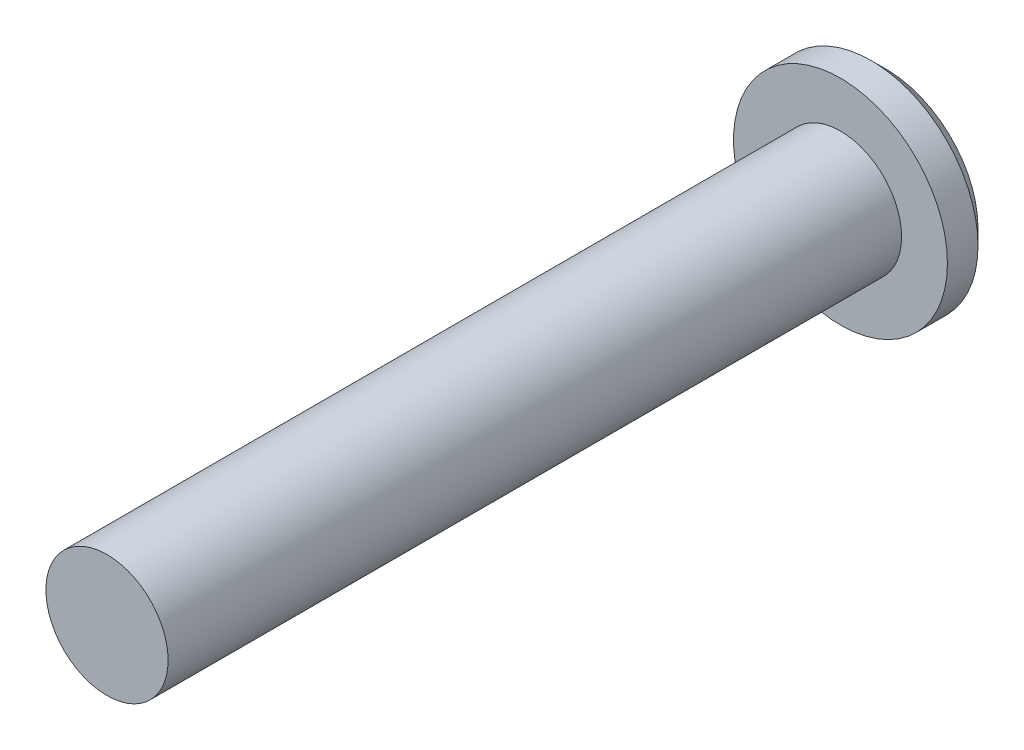
from build123d import *

# Parameters (mm, degrees)
HEAD_PROFILE_14_R      = 7
HEAD_14X3_DEPTH        = 3
SHANK_PROFILE_8_R      = 4
SHANK_8X48_DEPTH       = 48
HEAD_CHAMFER_1X45_SIZE = 1


with BuildPart() as part:
    # Head Profile Ø14 → Head Ø14x3 (new body)
    with BuildSketch(Plane.XY):
        Circle(HEAD_PROFILE_14_R)
    extrude(amount=HEAD_14X3_DEPTH)

    # Shank Profile Ø8 → Shank Ø8x48 (add)
    with BuildSketch(Plane.XY.offset(3)):
        Circle(SHANK_PROFILE_8_R)
    extrude(amount=SHANK_8X48_DEPTH)

    # Head Chamfer 1x45°
    head_chamfer_1x45_edges = [part.edges().sort_by_distance(p)[0] for p in [
        (-7, 0, 0),
    ]]
    chamfer(head_chamfer_1x45_edges, length=HEAD_CHAMFER_1X45_SIZE)


solid = part.part
